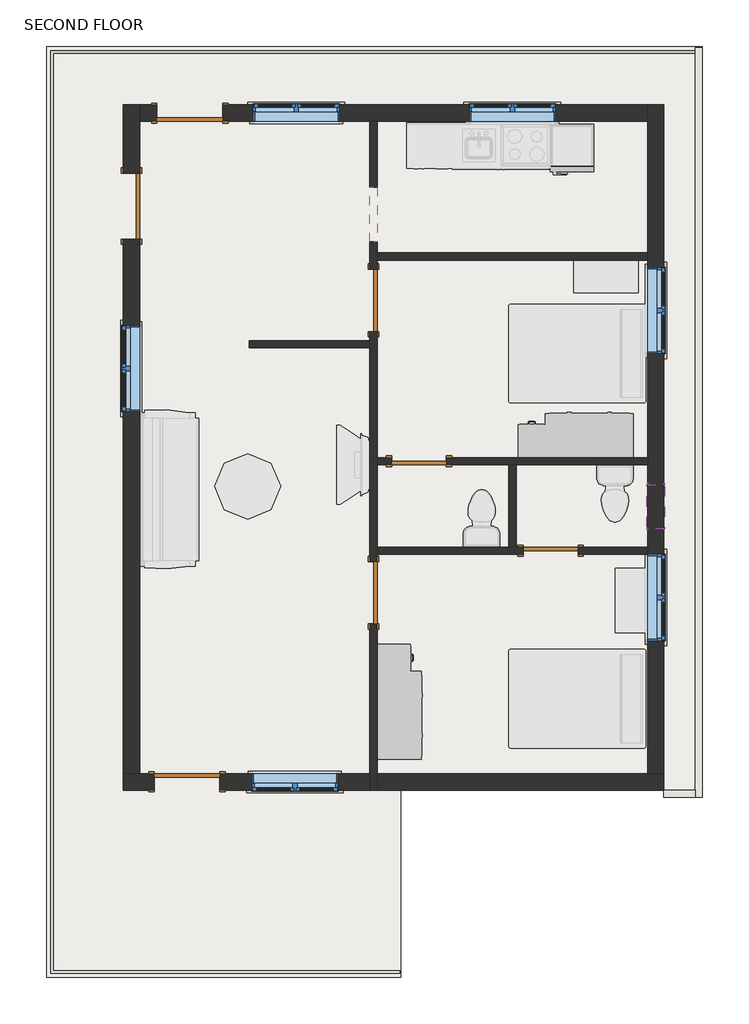
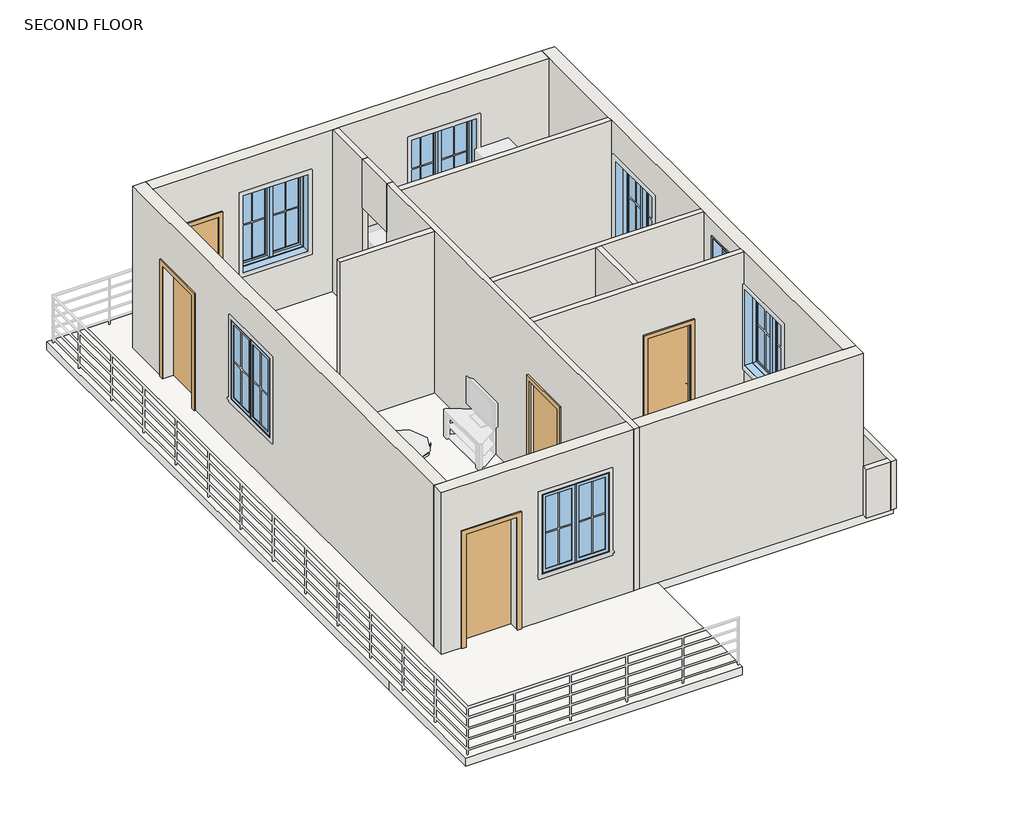
# One storey, part 1 of 3: 15 walls, 7 doors, 7 windows, 1 slab.
"""IFC4 building model written with IfcOpenShell, lengths in millimetres."""

from ifc_helpers import new_model, si_unit, frame, origin, place, context, project, spatial, polyline, outline, extrude, faceted_brep, transform, mapped, element, save
from components import m_single_flush_0762_x_2032mm_63ada305, m_single_flush_0762_x_2032mm_debabc81, m_single_flush_0864_x_2032mm_c62421c0, m_single_flush_0915_x_2134mm_43602619, m_single_flush_0915_x_2134mm_1ddf3370, m_window_casement_double_1200_x_1500mm_04159c99, window_f2d8fef0

model = new_model("IFC4")

# Units and contexts
model_context = context("Model", 3, world=origin())
ifc_project = project(units=[si_unit("LENGTHUNIT", "METRE", prefix="MILLI")], contexts=[model_context])

# Site, building, storey
site = spatial("IfcSite", under=ifc_project)
building = spatial("IfcBuilding", under=site)
storey = spatial("IfcBuildingStorey", under=building, Name="SECOND FLOOR", Elevation=6400.8)

# Doors
placement = place(None, origin())
m_single_flush_0762_x_2032mm_shape = m_single_flush_0762_x_2032mm_63ada305(model_context)
element("IfcDoor", 1, ObjectType="M_Single-Flush : 0762 x 2032mm", at=placement, inside=storey, context=model_context, shape_type="MappedRepresentation", body=[
    mapped(m_single_flush_0762_x_2032mm_shape, transform((2297.1455952, -1088.4648653, 6400.8), x_axis=(-1.0, 0.0, 0.0), y_axis=(0.0, -1.0, 0.0), z_axis=(0.0, 0.0, 1.0))),
])
m_single_flush_0762_x_2032mm_2_shape = m_single_flush_0762_x_2032mm_debabc81(model_context)
element("IfcDoor", 2, ObjectType="M_Single-Flush : 0762 x 2032mm", at=placement, inside=storey, context=model_context, shape_type="MappedRepresentation", body=[
    mapped(m_single_flush_0762_x_2032mm_2_shape, transform((466.7455952, 156.1351347, 6400.8), x_axis=(-1.0, 0.0, 0.0), y_axis=(0.0, -1.0, 0.0), z_axis=(0.0, 0.0, 1.0))),
])
m_single_flush_0864_x_2032mm_shape = m_single_flush_0864_x_2032mm_c62421c0(model_context)
element("IfcDoor", 3, ObjectType="M_Single-Flush : 0864 x 2032mm", at=placement, inside=storey, context=model_context, shape_type="MappedRepresentation", body=[
    mapped(m_single_flush_0864_x_2032mm_shape, transform((-165.0544048, 2391.3351347, 6400.8), x_axis=(0.0, 1.0, 0.0), y_axis=(-1.0, 0.0, 0.0), z_axis=(0.0, 0.0, 1.0))),
])
element("IfcDoor", 4, ObjectType="M_Single-Flush : 0864 x 2032mm", at=placement, inside=storey, context=model_context, shape_type="MappedRepresentation", body=[
    mapped(m_single_flush_0864_x_2032mm_shape, transform((-165.0544048, -1671.2648653, 6400.8), x_axis=(0.0, 1.0, 0.0), y_axis=(-1.0, 0.0, 0.0), z_axis=(0.0, 0.0, 1.0))),
])
m_single_flush_0915_x_2134mm_shape = m_single_flush_0915_x_2134mm_43602619(model_context)
element("IfcDoor", 5, ObjectType="M_Single-Flush : 0915 x 2134mm", at=placement, inside=storey, context=model_context, shape_type="MappedRepresentation", body=[
    mapped(m_single_flush_0915_x_2134mm_shape, transform((-3530.5544048, 3703.0351347, 6400.8), x_axis=(0.0, 1.0, 0.0), y_axis=(-1.0, 0.0, 0.0), z_axis=(0.0, 0.0, 1.0))),
])
element("IfcDoor", 6, ObjectType="M_Single-Flush : 0915 x 2134mm", at=placement, inside=storey, context=model_context, shape_type="MappedRepresentation", body=[
    mapped(m_single_flush_0915_x_2134mm_shape, transform((-2758.7544048, -4301.5648653, 6400.8), x_axis=(-1.0, 0.0, 0.0), y_axis=(0.0, -1.0, 0.0), z_axis=(0.0, 0.0, 1.0))),
])
m_single_flush_0915_x_2134mm_2_shape = m_single_flush_0915_x_2134mm_1ddf3370(model_context)
element("IfcDoor", 7, ObjectType="M_Single-Flush : 0915 x 2134mm", at=placement, inside=storey, context=model_context, shape_type="MappedRepresentation", body=[
    mapped(m_single_flush_0915_x_2134mm_2_shape, transform((-2718.7544048, 4994.8351347, 6400.8), x_axis=(-1.0, 0.0, 0.0), y_axis=(0.0, -1.0, 0.0), z_axis=(0.0, 0.0, 1.0))),
])

# Slab
element("IfcSlab", 8, ObjectType="6\" floor", at=placement, inside=storey, context=model_context, shape_type="SweptSolid", body=[
    extrude(outline(polyline([(4406.9455952, 5921.9351347), (4406.9455952, -4415.8648653), (215.9455952, -4415.8648653), (215.9455952, -7021.8741001), (-4711.6544048, -7021.8741001), (-4711.6544048, -4637.8294487), (-4711.6544048, 5921.9351347), (4406.9455952, 5921.9351347)])), frame((0.0, 0.0, 6248.4), z_axis=(0.0, 0.0, 1.0), x_axis=(1.0, 0.0, 0.0)), (0.0, 0.0, 1.0), 152.4),
])

# Walls
element("IfcWall", 9, ObjectType="4\" wall", at=placement, inside=storey, context=model_context, shape_type="Brep", body=[
    faceted_brep([(-215.8544048, 3204.1351347, 6400.8), (-215.8544048, 2823.3351347, 6400.8), (-215.8544048, 2823.3351347, 8432.8), (-215.8544048, 1959.3351347, 8432.8), (-215.8544048, 1959.3351347, 6400.8), (-215.8544048, 1832.5351347, 6400.8), (-215.8544048, 1730.9351347, 6400.8), (-215.8544048, -1239.2648653, 6400.8), (-215.8544048, -1239.2648653, 8432.8), (-215.8544048, -2103.2648653, 8432.8), (-215.8544048, -2103.2648653, 6400.8), (-215.8544048, -4187.2648653, 6400.8), (-215.8544048, -4415.8648653, 6400.8), (-215.8544048, -4415.8648653, 9448.8), (-215.8544048, -4187.2648653, 9448.8), (-215.8544048, 1730.9351347, 9448.8), (-215.8544048, 1832.5351347, 9448.8), (-215.8544048, 3204.1351347, 9448.8), (-215.8544048, 3204.1351347, 8534.4), (-114.2544048, 2823.3351347, 8432.8), (-114.2544048, 2823.3351347, 6400.8), (-114.2544048, 2950.1351347, 6400.8), (-114.2544048, 3051.7351347, 6400.8), (-114.2544048, 3204.1351347, 6400.8), (-114.2544048, 3204.1351347, 8534.4), (-114.2544048, 3204.1351347, 9448.8), (-114.2544048, 3051.7351347, 9448.8), (-114.2544048, 2950.1351347, 9448.8), (-114.2544048, 206.9351347, 9448.8), (-114.2544048, 105.3351347, 9448.8), (-114.2544048, -1037.6648653, 9448.8), (-114.2544048, -1139.2648653, 9448.8), (-114.2544048, -4187.2648653, 9448.8), (-114.2544048, -4415.8648653, 9448.8), (-114.2544048, -4415.8648653, 6400.8), (-114.2544048, -4187.2648653, 6400.8), (-114.2544048, -2103.2648653, 6400.8), (-114.2544048, -2103.2648653, 8432.8), (-114.2544048, -1239.2648653, 8432.8), (-114.2544048, -1239.2648653, 6400.8), (-114.2544048, -1139.2648653, 6400.8), (-114.2544048, -1037.6648653, 6400.8), (-114.2544048, 105.3351347, 6400.8), (-114.2544048, 206.9351347, 6400.8), (-114.2544048, 1959.3351347, 6400.8), (-114.2544048, 1959.3351347, 8432.8)], [[[0, 1, 2, 3, 4, 5, 6, 7, 8, 9, 10, 11, 12, 13, 14, 15, 16, 17, 18]], [[19, 20, 21, 22, 23, 24, 25, 26, 27, 28, 29, 30, 31, 32, 33, 34, 35, 36, 37, 38, 39, 40, 41, 42, 43, 44, 45]], [[34, 12, 11, 10, 36, 35]], [[23, 22, 21, 20, 1, 0]], [[44, 43, 42, 41, 40, 39, 7, 6, 5, 4]], [[17, 16, 15, 14, 13, 33, 32, 31, 30, 29, 28, 27, 26, 25]], [[0, 18, 17, 25, 24, 23]], [[13, 12, 34, 33]], [[8, 38, 37, 9]], [[9, 37, 36, 10]], [[4, 3, 45, 44]], [[3, 2, 19, 45]], [[2, 1, 20, 19]], [[38, 8, 7, 39]]]),
])
element("IfcWall", 10, ObjectType="4\" wall", at=placement, inside=storey, context=model_context, shape_type="Brep", body=[
    faceted_brep([(-114.2544048, -1139.2648653, 6400.8), (1916.1455952, -1139.2648653, 6400.8), (1916.1455952, -1139.2648653, 8432.8), (2678.1455952, -1139.2648653, 8432.8), (2678.1455952, -1139.2648653, 6400.8), (3644.9455952, -1139.2648653, 6400.8), (3644.9455952, -1139.2648653, 7300.8), (3644.9455952, -1139.2648653, 8800.8), (3644.9455952, -1139.2648653, 9448.8), (-114.2544048, -1139.2648653, 9448.8), (1916.1455952, -1037.6648653, 8432.8), (1916.1455952, -1037.6648653, 6400.8), (1816.1455952, -1037.6648653, 6400.8), (1714.5455952, -1037.6648653, 6400.8), (-114.2544048, -1037.6648653, 6400.8), (-114.2544048, -1037.6648653, 9448.8), (1714.5455952, -1037.6648653, 9448.8), (1816.1455952, -1037.6648653, 9448.8), (3644.9455952, -1037.6648653, 9448.8), (3644.9455952, -1037.6648653, 6400.8), (2678.1455952, -1037.6648653, 6400.8), (2678.1455952, -1037.6648653, 8432.8)], [[[0, 1, 2, 3, 4, 5, 6, 7, 8, 9]], [[10, 11, 12, 13, 14, 15, 16, 17, 18, 19, 20, 21]], [[20, 19, 5, 4]], [[14, 13, 12, 11, 1, 0]], [[9, 8, 18, 17, 16, 15]], [[8, 7, 6, 5, 19, 18]], [[0, 9, 15, 14]], [[2, 1, 11, 10]], [[3, 2, 10, 21]], [[4, 3, 21, 20]]]),
])
element("IfcWall", 11, ObjectType="4\" wall", at=placement, inside=storey, context=model_context, shape_type="Brep", body=[
    faceted_brep([(85.7455952, 206.9351347, 8432.8), (85.7455952, 206.9351347, 6400.8), (-114.2544048, 206.9351347, 6400.8), (-114.2544048, 206.9351347, 9448.8), (3644.9455952, 206.9351347, 9448.8), (3644.9455952, 206.9351347, 6400.8), (847.7455952, 206.9351347, 6400.8), (847.7455952, 206.9351347, 8432.8), (-114.2544048, 105.3351347, 6400.8), (85.7455952, 105.3351347, 6400.8), (85.7455952, 105.3351347, 8432.8), (847.7455952, 105.3351347, 8432.8), (847.7455952, 105.3351347, 6400.8), (1714.5455952, 105.3351347, 6400.8), (1816.1455952, 105.3351347, 6400.8), (3644.9455952, 105.3351347, 6400.8), (3644.9455952, 105.3351347, 9448.8), (1816.1455952, 105.3351347, 9448.8), (1714.5455952, 105.3351347, 9448.8), (-114.2544048, 105.3351347, 9448.8)], [[[0, 1, 2, 3, 4, 5, 6, 7]], [[8, 9, 10, 11, 12, 13, 14, 15, 16, 17, 18, 19]], [[6, 5, 15, 14, 13, 12]], [[2, 1, 9, 8]], [[4, 3, 19, 18, 17, 16]], [[5, 4, 16, 15]], [[3, 2, 8, 19]], [[10, 9, 1, 0]], [[11, 10, 0, 7]], [[12, 11, 7, 6]]]),
])
element("IfcWall", 12, ObjectType="4\" wall", at=placement, inside=storey, context=model_context, shape_type="SweptSolid", body=[
    extrude(outline(polyline([(-215.8544048, 1730.9351347), (-1892.2544048, 1730.9351347), (-1892.2544048, 1832.5351347), (-215.8544048, 1832.5351347), (-215.8544048, 1730.9351347)])), frame((0.0, 0.0, 6400.8), z_axis=(0.0, 0.0, 1.0), x_axis=(1.0, 0.0, 0.0)), (0.0, 0.0, 1.0), 3048.0),
])
element("IfcWall", 13, ObjectType="4\" wall", at=placement, inside=storey, context=model_context, shape_type="SweptSolid", body=[
    extrude(outline(polyline([(-114.2544048, 3051.7351347), (3644.9455952, 3051.7351347), (3644.9455952, 2950.1351347), (-114.2544048, 2950.1351347), (-114.2544048, 3051.7351347)])), frame((0.0, 0.0, 6400.8), z_axis=(0.0, 0.0, 1.0), x_axis=(1.0, 0.0, 0.0)), (0.0, 0.0, 1.0), 3048.0),
])
element("IfcWall", 14, ObjectType="4\" wall", at=placement, inside=storey, context=model_context, shape_type="SweptSolid", body=[
    extrude(outline(polyline([(1714.5455952, -1037.6648653), (1714.5455952, 105.3351347), (1816.1455952, 105.3351347), (1816.1455952, -1037.6648653), (1714.5455952, -1037.6648653)])), frame((0.0, 0.0, 6400.8), z_axis=(0.0, 0.0, 1.0), x_axis=(1.0, 0.0, 0.0)), (0.0, 0.0, 1.0), 3048.0),
])
element("IfcWall", 15, ObjectType="4\" wall", at=placement, inside=storey, context=model_context, shape_type="Brep", body=[
    faceted_brep([(-215.8544048, 4880.5351347, 6400.8), (-215.8544048, 3966.1351347, 6400.8), (-215.8544048, 3966.1351347, 8534.4), (-215.8544048, 3966.1351347, 9448.8), (-215.8544048, 4880.5351347, 9448.8), (-114.2544048, 4880.5351347, 6400.8), (-114.2544048, 4880.5351347, 9448.8), (-114.2544048, 3966.1351347, 9448.8), (-114.2544048, 3966.1351347, 8534.4), (-114.2544048, 3966.1351347, 6400.8)], [[[0, 1, 2, 3, 4]], [[5, 6, 7, 8, 9]], [[1, 0, 5, 9]], [[3, 2, 1, 9, 8, 7]], [[4, 3, 7, 6]], [[0, 4, 6, 5]]]),
])
element("IfcWall", 16, ObjectType="4\" wall", at=placement, inside=storey, context=model_context, shape_type="SweptSolid", body=[
    extrude(outline(polyline([(-215.8544048, 3204.1351347), (-215.8544048, 3966.1351347), (-114.2544048, 3966.1351347), (-114.2544048, 3204.1351347), (-215.8544048, 3204.1351347)])), frame((0.0, 0.0, 8534.4), z_axis=(0.0, 0.0, 1.0), x_axis=(1.0, 0.0, 0.0)), (0.0, 0.0, 1.0), 914.4),
])
element("IfcWall", 17, ObjectType="4\" wall", at=placement, inside=storey, context=model_context, shape_type="Brep", body=[
    faceted_brep([(4305.3455952, 5901.9351347, 6400.8), (4305.3455952, -4415.8648653, 6400.8), (4305.3455952, -4517.4648653, 6400.8), (4305.3455952, -4517.4648653, 7315.2), (4305.3455952, -4415.8648653, 7315.2), (4305.3455952, 5901.9351347, 7315.2), (4406.9455952, 5901.9351347, 6400.8), (4406.9455952, 5901.9351347, 7315.2), (4406.9455952, -4517.4648653, 7315.2), (4406.9455952, -4517.4648653, 6400.8)], [[[0, 1, 2, 3, 4, 5]], [[6, 7, 8, 9]], [[2, 1, 0, 6, 9]], [[5, 4, 3, 8, 7]], [[0, 5, 7, 6]], [[3, 2, 9, 8]]]),
])
element("IfcWall", 18, ObjectType="4\" wall", at=placement, inside=storey, context=model_context, shape_type="SweptSolid", body=[
    extrude(outline(polyline([(3873.5455952, -4415.8648653), (4305.3455952, -4415.8648653), (4305.3455952, -4517.4648653), (3873.5455952, -4517.4648653), (3873.5455952, -4415.8648653)])), frame((0.0, 0.0, 6400.8), z_axis=(0.0, 0.0, 1.0), x_axis=(1.0, 0.0, 0.0)), (0.0, 0.0, 1.0), 914.4),
])
element("IfcWall", 19, ObjectType="9\" wall", at=placement, inside=storey, context=model_context, shape_type="Brep", body=[
    faceted_brep([(-3644.8544048, 5109.1351347, 6400.8), (-3644.8544048, 4160.5351347, 6400.8), (-3644.8544048, 4160.5351347, 8534.8), (-3644.8544048, 3245.5351347, 8534.8), (-3644.8544048, 3245.5351347, 6400.8), (-3644.8544048, -4187.2648653, 6400.8), (-3644.8544048, -4187.2648653, 9448.8), (-3644.8544048, 5109.1351347, 9448.8), (-3644.8544048, 2045.5351347, 8800.8), (-3644.8544048, 845.5351347, 8800.8), (-3644.8544048, 845.5351347, 7300.8), (-3644.8544048, 2045.5351347, 7300.8), (-3416.2544048, 4160.5351347, 8534.8), (-3416.2544048, 4160.5351347, 6400.8), (-3416.2544048, 4880.5351347, 6400.8), (-3416.2544048, 5109.1351347, 6400.8), (-3416.2544048, 5109.1351347, 9448.8), (-3416.2544048, 4880.5351347, 9448.8), (-3416.2544048, -4187.2648653, 9448.8), (-3416.2544048, -4187.2648653, 6400.8), (-3416.2544048, 3245.5351347, 6400.8), (-3416.2544048, 3245.5351347, 8534.8), (-3416.2544048, 2045.5351347, 8800.8), (-3416.2544048, 2045.5351347, 7300.8), (-3416.2544048, 845.5351347, 7300.8), (-3416.2544048, 845.5351347, 8800.8)], [[[0, 1, 2, 3, 4, 5, 6, 7], [8, 9, 10, 11]], [[12, 13, 14, 15, 16, 17, 18, 19, 20, 21], [22, 23, 24, 25]], [[20, 19, 5, 4]], [[15, 14, 13, 1, 0]], [[7, 6, 18, 17, 16]], [[0, 7, 16, 15]], [[2, 1, 13, 12]], [[3, 2, 12, 21]], [[4, 3, 21, 20]], [[23, 22, 8, 11]], [[24, 23, 11, 10]], [[25, 24, 10, 9]], [[22, 25, 9, 8]], [[6, 5, 19, 18]]]),
])
element("IfcWall", 20, ObjectType="9\" wall", at=placement, inside=storey, context=model_context, shape_type="Brep", body=[
    faceted_brep([(-114.2544048, -4415.8648653, 6400.8), (3873.5455952, -4415.8648653, 6400.8), (3873.5455952, -4415.8648653, 9448.8), (-114.2544048, -4415.8648653, 9448.8), (-114.2544048, -4187.2648653, 6400.8), (-114.2544048, -4187.2648653, 9448.8), (3644.9455952, -4187.2648653, 9448.8), (3873.5455952, -4187.2648653, 9448.8), (3873.5455952, -4187.2648653, 6400.8), (3644.9455952, -4187.2648653, 6400.8)], [[[0, 1, 2, 3]], [[4, 5, 6, 7, 8, 9]], [[1, 0, 4, 9, 8]], [[3, 2, 7, 6, 5]], [[0, 3, 5, 4]], [[2, 1, 8, 7]]]),
])
element("IfcWall", 21, ObjectType="9\" wall", at=placement, inside=storey, context=model_context, shape_type="Brep", body=[
    faceted_brep([(3873.5455952, -4187.2648653, 6400.8), (3873.5455952, 5109.1351347, 6400.8), (3873.5455952, 5109.1351347, 9448.8), (3873.5455952, -4187.2648653, 9448.8), (3873.5455952, 1650.1351347, 8800.8), (3873.5455952, 2850.1351347, 8800.8), (3873.5455952, 2850.1351347, 7300.8), (3873.5455952, 1650.1351347, 7300.8), (3873.5455952, -2339.2648653, 8800.8), (3873.5455952, -1139.2648653, 8800.8), (3873.5455952, -1139.2648653, 7300.8), (3873.5455952, -2339.2648653, 7300.8), (3873.5455952, -170.8898653, 9144.0), (3873.5455952, -170.8898653, 8534.4), (3873.5455952, -780.4898653, 8534.4), (3873.5455952, -780.4898653, 9144.0), (3644.9455952, -4187.2648653, 6400.8), (3644.9455952, -4187.2648653, 9448.8), (3644.9455952, -1139.2648653, 9448.8), (3644.9455952, -1037.6648653, 9448.8), (3644.9455952, 105.3351347, 9448.8), (3644.9455952, 206.9351347, 9448.8), (3644.9455952, 2950.1351347, 9448.8), (3644.9455952, 3051.7351347, 9448.8), (3644.9455952, 4880.5351347, 9448.8), (3644.9455952, 5109.1351347, 9448.8), (3644.9455952, 5109.1351347, 6400.8), (3644.9455952, 4880.5351347, 6400.8), (3644.9455952, 3051.7351347, 6400.8), (3644.9455952, 2950.1351347, 6400.8), (3644.9455952, 206.9351347, 6400.8), (3644.9455952, 105.3351347, 6400.8), (3644.9455952, -1037.6648653, 6400.8), (3644.9455952, -1139.2648653, 6400.8), (3644.9455952, 1650.1351347, 8800.8), (3644.9455952, 1650.1351347, 7300.8), (3644.9455952, 2850.1351347, 7300.8), (3644.9455952, 2850.1351347, 8800.8), (3644.9455952, -2339.2648653, 8800.8), (3644.9455952, -2339.2648653, 7300.8), (3644.9455952, -1139.2648653, 7300.8), (3644.9455952, -1139.2648653, 8800.8), (3644.9455952, -170.8898653, 9144.0), (3644.9455952, -780.4898653, 9144.0), (3644.9455952, -780.4898653, 8534.4), (3644.9455952, -170.8898653, 8534.4)], [[[0, 1, 2, 3], [4, 5, 6, 7], [8, 9, 10, 11], [12, 13, 14, 15]], [[16, 17, 18, 19, 20, 21, 22, 23, 24, 25, 26, 27, 28, 29, 30, 31, 32, 33], [34, 35, 36, 37], [38, 39, 40, 41], [42, 43, 44, 45]], [[1, 0, 16, 33, 32, 31, 30, 29, 28, 27, 26]], [[3, 2, 25, 24, 23, 22, 21, 20, 19, 18, 17]], [[0, 3, 17, 16]], [[2, 1, 26, 25]], [[35, 34, 4, 7]], [[36, 35, 7, 6]], [[37, 36, 6, 5]], [[34, 37, 5, 4]], [[39, 38, 8, 11]], [[40, 39, 11, 10]], [[41, 40, 10, 9]], [[38, 41, 9, 8]], [[13, 12, 42, 45]], [[14, 13, 45, 44]], [[15, 14, 44, 43]], [[12, 15, 43, 42]]]),
])
element("IfcWall", 22, ObjectType="9\" wall", at=placement, inside=storey, context=model_context, shape_type="Brep", body=[
    faceted_brep([(-3176.2544048, 5109.1351347, 8534.8), (-3176.2544048, 5109.1351347, 6400.8), (-3416.2544048, 5109.1351347, 6400.8), (-3416.2544048, 5109.1351347, 9448.8), (3644.9455952, 5109.1351347, 9448.8), (3644.9455952, 5109.1351347, 6400.8), (-2261.2544048, 5109.1351347, 6400.8), (-2261.2544048, 5109.1351347, 8534.8), (2365.3455952, 5109.1351347, 8800.8), (1165.3455952, 5109.1351347, 8800.8), (1165.3455952, 5109.1351347, 7300.8), (2365.3455952, 5109.1351347, 7300.8), (-638.5544048, 5109.1351347, 8800.8), (-1838.5544048, 5109.1351347, 8800.8), (-1838.5544048, 5109.1351347, 7300.8), (-638.5544048, 5109.1351347, 7300.8), (-3416.2544048, 4880.5351347, 6400.8), (-3176.2544048, 4880.5351347, 6400.8), (-3176.2544048, 4880.5351347, 8534.8), (-2261.2544048, 4880.5351347, 8534.8), (-2261.2544048, 4880.5351347, 6400.8), (-215.8544048, 4880.5351347, 6400.8), (-114.2544048, 4880.5351347, 6400.8), (3644.9455952, 4880.5351347, 6400.8), (3644.9455952, 4880.5351347, 9448.8), (-114.2544048, 4880.5351347, 9448.8), (-215.8544048, 4880.5351347, 9448.8), (-3416.2544048, 4880.5351347, 9448.8), (2365.3455952, 4880.5351347, 8800.8), (2365.3455952, 4880.5351347, 7300.8), (1165.3455952, 4880.5351347, 7300.8), (1165.3455952, 4880.5351347, 8800.8), (-638.5544048, 4880.5351347, 8800.8), (-638.5544048, 4880.5351347, 7300.8), (-1838.5544048, 4880.5351347, 7300.8), (-1838.5544048, 4880.5351347, 8800.8)], [[[0, 1, 2, 3, 4, 5, 6, 7], [8, 9, 10, 11], [12, 13, 14, 15]], [[16, 17, 18, 19, 20, 21, 22, 23, 24, 25, 26, 27], [28, 29, 30, 31], [32, 33, 34, 35]], [[6, 5, 23, 22, 21, 20]], [[2, 1, 17, 16]], [[4, 3, 27, 26, 25, 24]], [[5, 4, 24, 23]], [[3, 2, 16, 27]], [[18, 17, 1, 0]], [[19, 18, 0, 7]], [[20, 19, 7, 6]], [[29, 28, 8, 11]], [[30, 29, 11, 10]], [[31, 30, 10, 9]], [[28, 31, 9, 8]], [[33, 32, 12, 15]], [[34, 33, 15, 14]], [[35, 34, 14, 13]], [[32, 35, 13, 12]]]),
])
element("IfcWall", 23, ObjectType="9\" wall", at=placement, inside=storey, context=model_context, shape_type="Brep", body=[
    faceted_brep([(-3644.8544048, -4415.8648653, 6400.8), (-3216.2544048, -4415.8648653, 6400.8), (-3216.2544048, -4415.8648653, 8534.8), (-2301.2544048, -4415.8648653, 8534.8), (-2301.2544048, -4415.8648653, 6400.8), (-215.8544048, -4415.8648653, 6400.8), (-215.8544048, -4415.8648653, 9448.8), (-3644.8544048, -4415.8648653, 9448.8), (-1858.5544048, -4415.8648653, 8800.8), (-658.5544048, -4415.8648653, 8800.8), (-658.5544048, -4415.8648653, 7300.8), (-1858.5544048, -4415.8648653, 7300.8), (-3216.2544048, -4187.2648653, 8534.8), (-3216.2544048, -4187.2648653, 6400.8), (-3416.2544048, -4187.2648653, 6400.8), (-3644.8544048, -4187.2648653, 6400.8), (-3644.8544048, -4187.2648653, 9448.8), (-3416.2544048, -4187.2648653, 9448.8), (-215.8544048, -4187.2648653, 9448.8), (-215.8544048, -4187.2648653, 6400.8), (-2301.2544048, -4187.2648653, 6400.8), (-2301.2544048, -4187.2648653, 8534.8), (-1858.5544048, -4187.2648653, 8800.8), (-1858.5544048, -4187.2648653, 7300.8), (-658.5544048, -4187.2648653, 7300.8), (-658.5544048, -4187.2648653, 8800.8)], [[[0, 1, 2, 3, 4, 5, 6, 7], [8, 9, 10, 11]], [[12, 13, 14, 15, 16, 17, 18, 19, 20, 21], [22, 23, 24, 25]], [[20, 19, 5, 4]], [[15, 14, 13, 1, 0]], [[7, 6, 18, 17, 16]], [[2, 1, 13, 12]], [[3, 2, 12, 21]], [[4, 3, 21, 20]], [[23, 22, 8, 11]], [[24, 23, 11, 10]], [[25, 24, 10, 9]], [[22, 25, 9, 8]], [[6, 5, 19, 18]], [[0, 7, 16, 15]]]),
])

# Windows
m_window_casement_double_1200_x_1500mm_shape = m_window_casement_double_1200_x_1500mm_04159c99(model_context)
element("IfcWindow", 24, ObjectType="M_Window-Casement-Double : 1200 x 1500mm", at=placement, inside=storey, context=model_context, shape_type="MappedRepresentation", body=[
    mapped(m_window_casement_double_1200_x_1500mm_shape, transform((1765.3455952, 4994.8351347, 6400.8), x_axis=(1.0, 0.0, 0.0), y_axis=(0.0, 1.0, 0.0), z_axis=(0.0, 0.0, 1.0))),
])
element("IfcWindow", 25, ObjectType="M_Window-Casement-Double : 1200 x 1500mm", at=placement, inside=storey, context=model_context, shape_type="MappedRepresentation", body=[
    mapped(m_window_casement_double_1200_x_1500mm_shape, transform((3759.2455952, 2250.1351347, 6400.8), x_axis=(0.0, -1.0, 0.0), y_axis=(1.0, 0.0, 0.0), z_axis=(0.0, 0.0, 1.0))),
])
element("IfcWindow", 26, ObjectType="M_Window-Casement-Double : 1200 x 1500mm", at=placement, inside=storey, context=model_context, shape_type="MappedRepresentation", body=[
    mapped(m_window_casement_double_1200_x_1500mm_shape, transform((3759.2455952, -1739.2648653, 6400.8), x_axis=(0.0, -1.0, 0.0), y_axis=(1.0, 0.0, 0.0), z_axis=(0.0, 0.0, 1.0))),
])
element("IfcWindow", 27, ObjectType="M_Window-Casement-Double : 1200 x 1500mm", at=placement, inside=storey, context=model_context, shape_type="MappedRepresentation", body=[
    mapped(m_window_casement_double_1200_x_1500mm_shape, transform((-3530.5544048, 1445.5351347, 6400.8), x_axis=(0.0, 1.0, 0.0), y_axis=(-1.0, 0.0, 0.0), z_axis=(0.0, 0.0, 1.0))),
])
element("IfcWindow", 28, ObjectType="M_Window-Casement-Double : 1200 x 1500mm", at=placement, inside=storey, context=model_context, shape_type="MappedRepresentation", body=[
    mapped(m_window_casement_double_1200_x_1500mm_shape, transform((-1238.5544048, 4994.8351347, 6400.8), x_axis=(1.0, 0.0, 0.0), y_axis=(0.0, 1.0, 0.0), z_axis=(0.0, 0.0, 1.0))),
])
element("IfcWindow", 29, ObjectType="M_Window-Casement-Double : 1200 x 1500mm", at=placement, inside=storey, context=model_context, shape_type="MappedRepresentation", body=[
    mapped(m_window_casement_double_1200_x_1500mm_shape, transform((-1258.5544048, -4301.5648653, 6400.8), x_axis=(-1.0, 0.0, 0.0), y_axis=(0.0, -1.0, 0.0), z_axis=(0.0, 0.0, 1.0))),
])
window_shape = window_f2d8fef0(model_context)
element("IfcWindow", 30, ObjectType="Window-Louvers : 24\" x 24\"", at=placement, inside=storey, context=model_context, shape_type="MappedRepresentation", body=[
    mapped(window_shape, transform((3765.5955952, -475.6898653, 7620.0), x_axis=(0.0, -1.0, 0.0), y_axis=(1.0, 0.0, 0.0), z_axis=(0.0, 0.0, 1.0))),
])

save(model, "model.ifc")

# Revit data of these elements
# Type "M_Single-Flush : 0762 x 2032mm"
#   Type Mark = "28"
#   Construction Type Id = "MDOOR"
#   Analytic Construction = "Metal"
#   Thickness = 0.167323 ft
#   Thermal Resistance (R) = 0.270117 (m²·K)/W
#   Heat Transfer Coefficient (U) = 3.7021 W/(m²·K)
#   Height = 6.666667 ft
#   Trim Projection Ext = 0.082021 ft
#   Trim Projection Int = 0.082021 ft
#   Trim Width = 0.249344 ft
#   Width = 2.5 ft
#   Define Thermal Properties by = 1
#   Define Thermal Properties by = 1
#   Door Material = Door - Panel
#   Frame Material = Door - Frame
#   Visual Light Transmittance = 0
#   Solar Heat Gain Coefficient = 0
#   Function = (empty or 0)
#   Wall Closure = (empty or 0)
# Type "M_Single-Flush : 0864 x 2032mm"
#   Type Mark = "32"
#   Construction Type Id = "MDOOR"
#   Analytic Construction = "Metal"
#   Thickness = 0.167323 ft
#   Thermal Resistance (R) = 0.270117 (m²·K)/W
#   Heat Transfer Coefficient (U) = 3.7021 W/(m²·K)
#   Height = 6.666667 ft
#   Trim Projection Ext = 0.082021 ft
#   Trim Projection Int = 0.082021 ft
#   Trim Width = 0.249344 ft
#   Width = 2.834646 ft
#   Define Thermal Properties by = 1
#   Define Thermal Properties by = 1
#   Door Material = Door - Panel
#   Frame Material = Door - Frame
#   Visual Light Transmittance = 0
#   Solar Heat Gain Coefficient = 0
#   Function = (empty or 0)
#   Wall Closure = (empty or 0)
# Type "M_Single-Flush : 0915 x 2134mm"
#   Type Mark = "20"
#   Construction Type Id = "MDOOR"
#   Analytic Construction = "Metal"
#   Thickness = 0.167323 ft
#   Thermal Resistance (R) = 0.270117 (m²·K)/W
#   Heat Transfer Coefficient (U) = 3.7021 W/(m²·K)
#   Height = 7.001312 ft
#   Trim Projection Ext = 0.082021 ft
#   Trim Projection Int = 0.082021 ft
#   Trim Width = 0.249344 ft
#   Width = 3.001969 ft
#   Define Thermal Properties by = 1
#   Define Thermal Properties by = 1
#   Door Material = Door - Panel
#   Frame Material = Door - Frame
#   Visual Light Transmittance = 0
#   Solar Heat Gain Coefficient = 0
#   Function = (empty or 0)
#   Wall Closure = (empty or 0)
# Type "6\" floor"
#   Function = 0
#   Layers, outside or top first: 0.5 ft no material (function 1)
# Type "4\" wall"
#   Layers, outside or top first: 0.333333 ft no material (function 1)
# Type "9\" wall"
#   Layers, outside or top first: 0.75 ft no material (function 1)
# Type "M_Window-Casement-Double : 1200 x 1500mm"
#   Type Mark = "25"
#   Fire Rating = "0.5h"
#   Assembly Code = "B2020100"
#   Analytic Construction = "Double glazing - domestic"
#   Frame Extension [instance default] = 0.020833 ft
#   Window Inset [instance default] = 0.0 ft
#   Wall Thickness [instance default] = 0.492126 ft
#   Interior Wall Closure [instance default] = 0.179626 ft
#   Half Width = 1.968504 ft
#   Visual Light Transmittance = 0.81
#   Thermal Resistance (R) = 0.319569 (m²·K)/W
#   Solar Heat Gain Coefficient = 0.76
#   Rough Width = 3.98622 ft
#   Rough Height = 4.970472 ft
#   Height = 4.92126 ft
#   Heat Transfer Coefficient (U) = 3.12929 W/(m²·K)
#   Exterior Wall Closure [instance default] = 0.104331 ft
#   Extension Jamb [instance default] = 0.179626 ft
#   Default Sill Height = 2.952756 ft
#   Width = 3.937008 ft
#   Define Thermal Properties by = 0
#   Muntin Visibility = yes
#   Interior Trim Visibility [instance default] = yes
#   Exterior Trim Visibility [instance default] = yes
#   Extension Jamb Visibility [instance default] = yes
#   Interior Trim Material = Wood - Stained
#   Muntin Pattern = M_Muntin Pattern_2x2 : M_Muntin Pattern_2x2
#   Interior Trim = M_Trim-Window-Interior-Flat : Picture Frame
#   Interior Frame Material = Wood - Stained
#   Glass Panel Material = Glass
#   Exterior Trim Material = Clad - White
#   Exterior Trim = M_Trim-Window-Exterior-Flat : with Sill
#   Exterior Frame Material = Clad - White
#   Wall Closure = (empty or 0)
# Type "Window-Louvers : 24\" x 24\""
#   Type Mark = "28"
#   Construction Type Id = "GSP4R"
#   Assembly Code = "B20"
#   Analytic Construction = "1/8 in Pilkington single glazing"
#   Visual Light Transmittance = 0.9
#   Thermal Resistance (R) = 0.271106 (m²·K)/W
#   Solar Heat Gain Coefficient = 0.78
#   Max Height = 1.978553 ft
#   Height = 2.0 ft
#   Heat Transfer Coefficient (U) = 3.6886 W/(m²·K)
#   Blade Width [instance default] = 1.875 ft
#   Blade Vertical Thickness = 0.029463 ft
#   Blade Thickness = 0.020833 ft
#   Blade Spacing = 0.125 ft
#   Blade Height = 0.154463 ft
#   Blade Depth = 0.25 ft
#   Blade Angle = 45.00°
#   Default Sill Height = 3.0 ft
#   Trim Projection_Exterior = 0.041667 ft
#   Trim Projection_Interior = 0.041667 ft
#   Trim Width_Exterior = 0.125 ft
#   Trim Width_Interior = 0.125 ft
#   Width = 2.0 ft
#   Max Blade Count = 12
#   Define Thermal Properties by = 1
#   Blade Count = 12
#   Frame Material = Birch
#   Louver Material = Birch
#   Trim Exterior Material = Birch
#   Trim Interior Material = Birch
#   Wall Closure = (empty or 0)
# Elements 1, 2 (IfcDoor, "M_Single-Flush : 0762 x 2032mm")
#   Phase Created = New Construction
#   Materials on its faces: "Door - Frame", "Door - Panel"
# Elements 3, 4 (IfcDoor, "M_Single-Flush : 0864 x 2032mm")
#   Phase Created = New Construction
#   Materials on its faces: "Door - Frame", "Door - Panel"
# Elements 5, 6, 7 (IfcDoor, "M_Single-Flush : 0915 x 2134mm")
#   Phase Created = New Construction
#   Materials on its faces: "Door - Frame", "Door - Panel"
# Element 8 (IfcSlab, "6\" floor")
#   Height Offset From Level = 0.0 ft
#   Phase Created = New Construction
#   Materials on its faces: "Default Floor"
# Elements 9, 10, 11, 12, 13, 14, 15 (IfcWall, "4\" wall")
#   Top Offset = 0.0 ft
#   Base Offset = 0.0 ft
#   Unconnected Height = 10.0 ft
#   wall height = 10.0 ft
#   Phase Created = New Construction
#   Base Constraint = SECOND FLOOR
#   Materials on its faces: "Default Wall"
# Element 16 (IfcWall, "4\" wall")
#   built-in parameter 1001111 = 7.0 ft
#   Top Offset = 0.0 ft
#   Base Offset = 7.0 ft
#   Unconnected Height = 3.0 ft
#   wall height = 3.0 ft
#   Phase Created = New Construction
#   Base Constraint = SECOND FLOOR
#   Materials on its faces: "Default Wall"
# Elements 17, 18 (IfcWall, "4\" wall")
#   Top Offset = 0.0 ft
#   Base Offset = 0.0 ft
#   Unconnected Height = 3.0 ft
#   wall height = 3.0 ft
#   Phase Created = New Construction
#   Base Constraint = SECOND FLOOR
#   Materials on its faces: "Default Wall"
# Elements 19, 20, 21, 22, 23 (IfcWall, "9\" wall")
#   Top Offset = 0.0 ft
#   Base Offset = 0.0 ft
#   Unconnected Height = 10.0 ft
#   wall height = 10.0 ft
#   Phase Created = New Construction
#   Base Constraint = SECOND FLOOR
#   Materials on its faces: "Default Wall"
# Element 24 (IfcWindow, "M_Window-Casement-Double : 1200 x 1500mm")
#   Mark = "15"
#   Window Inset = 0.0 ft
#   Interior Wall Closure = 0.179626 ft
#   Frame Extension = 0.020833 ft
#   Exterior Wall Closure = 0.104331 ft
#   Interior Trim Visibility = yes
#   Exterior Trim Visibility = yes
#   Phase Created = New Construction
#   Materials on its faces: "Wood - Stained", "Glass", "Clad - White"
# Element 25 (IfcWindow, "M_Window-Casement-Double : 1200 x 1500mm")
#   Mark = "16"
#   Window Inset = 0.0 ft
#   Interior Wall Closure = 0.179626 ft
#   Frame Extension = 0.020833 ft
#   Exterior Wall Closure = 0.104331 ft
#   Interior Trim Visibility = yes
#   Exterior Trim Visibility = yes
#   Phase Created = New Construction
#   Materials on its faces: "Wood - Stained", "Glass", "Clad - White"
# Element 26 (IfcWindow, "M_Window-Casement-Double : 1200 x 1500mm")
#   Mark = "17"
#   Window Inset = 0.0 ft
#   Interior Wall Closure = 0.179626 ft
#   Frame Extension = 0.020833 ft
#   Exterior Wall Closure = 0.104331 ft
#   Interior Trim Visibility = yes
#   Exterior Trim Visibility = yes
#   Phase Created = New Construction
#   Materials on its faces: "Wood - Stained", "Glass", "Clad - White"
# Element 27 (IfcWindow, "M_Window-Casement-Double : 1200 x 1500mm")
#   Mark = "19"
#   Window Inset = 0.0 ft
#   Interior Wall Closure = 0.179626 ft
#   Frame Extension = 0.020833 ft
#   Exterior Wall Closure = 0.104331 ft
#   Interior Trim Visibility = yes
#   Exterior Trim Visibility = yes
#   Phase Created = New Construction
#   Materials on its faces: "Wood - Stained", "Glass", "Clad - White"
# Element 28 (IfcWindow, "M_Window-Casement-Double : 1200 x 1500mm")
#   Mark = "20"
#   Window Inset = 0.0 ft
#   Interior Wall Closure = 0.179626 ft
#   Frame Extension = 0.020833 ft
#   Exterior Wall Closure = 0.104331 ft
#   Interior Trim Visibility = yes
#   Exterior Trim Visibility = yes
#   Phase Created = New Construction
#   Materials on its faces: "Wood - Stained", "Glass", "Clad - White"
# Element 29 (IfcWindow, "M_Window-Casement-Double : 1200 x 1500mm")
#   Mark = "23"
#   Window Inset = 0.0 ft
#   Interior Wall Closure = 0.179626 ft
#   Frame Extension = 0.020833 ft
#   Exterior Wall Closure = 0.104331 ft
#   Interior Trim Visibility = yes
#   Exterior Trim Visibility = yes
#   Phase Created = New Construction
#   Materials on its faces: "Wood - Stained", "Glass", "Clad - White"
# Element 30 (IfcWindow, "Window-Louvers : 24\" x 24\"")
#   Mark = "21"
#   Blade Width = 1.875 ft
#   Phase Created = New Construction
#   Materials on its faces: "Birch"
# Materials
#   "Door - Panel": class "Wood", colour RGB 210 159 95, transparency 0, Cost = 0
#   "Door - Frame": colour RGB 118 70 51, transparency 0, Cost = 0
#   "Wood - Stained": class "Wood", colour RGB 224 178 126, transparency 0, Cost = 0
#   "Glass": class "Glass", colour RGB 0 128 192, transparency 0.9, Description = "Soda Lime Glass", Cost = 0
#   "Clad - White": class "Wood", colour RGB 242 242 238, transparency 0, Cost = 0
#   "Birch": class "Wood", colour RGB 224 178 126, transparency 0, Description = "Betula Alleghaniensis", Cost = 0
#   "Default Floor": colour RGB 127 127 127, transparency 0, Cost = 0
#   "Default Wall": colour RGB 128 128 128, transparency 0, Cost = 0
